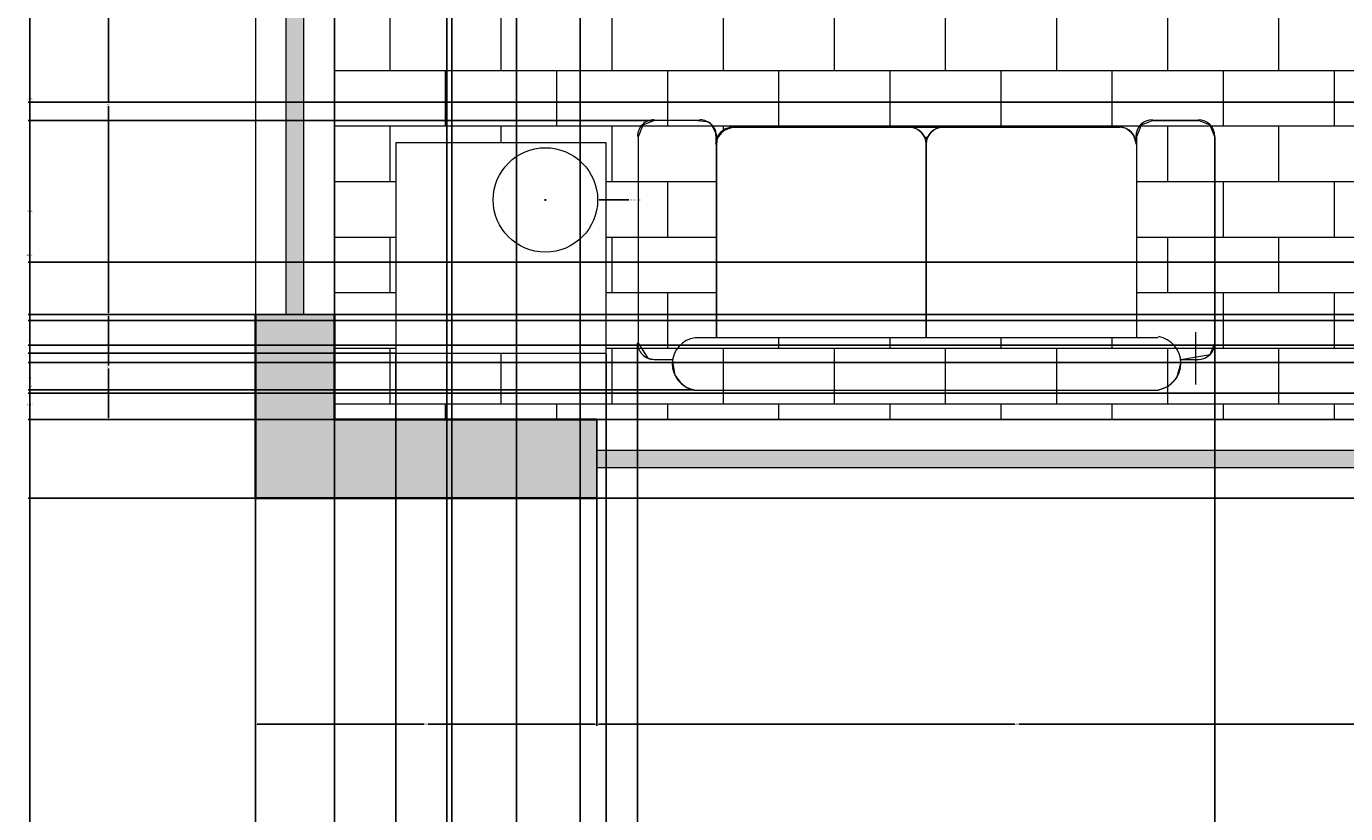
# Model space of a CAD drawing. Units: inches. Extents: x 6 to 575, y 34 to 566.
# Tile 2 of 21: x 6 to 157, y 168 to 258. Entities that reach past the tile are written whole.
import ezdxf

# ---------------------------------------------------------------- set-up
doc = ezdxf.new("R2010")
doc.units = ezdxf.units.IN
for name, color, linetype, lineweight in [('A-ANNO-DIMS', 2, 'Continuous', 18), ('A-FLOR-PATT', 252, 'Continuous', 9), ('A-GLAZ-PATT', 4, 'Continuous', 9), ('A-WALL-PATT', 251, 'Continuous', 9), ('FUR', 2, 'Continuous', 18), ('WALLS', 7, 'Continuous', 35), ('WINDOWS', 4, 'Continuous', 20)]:
    doc.layers.add(name, color=color, linetype=linetype, lineweight=lineweight)
doc.styles.get("Standard").update_dxf_attribs({"font": 'arial.ttf'})
doc.dimstyles.get("Standard").update_dxf_attribs({"dimtxt": 0.18, "dimasz": 0.18, "dimexe": 0.18, "dimexo": 0.0625, "dimgap": 0.09, "dimtad": 0, "dimtih": 1, "dimtoh": 1, "dimdec": 4, "dimzin": 0, "dimdsep": 46, "dimtxsty": 'Standard', "dimcen": 0.09, "dimadec": 0, "dimazin": 0, "dimtfac": 1, "dimtdec": 4, "dimtofl": 0, "dimtmove": 0, "dimatfit": 3, "dimfxl": 1, "dimtolj": 1, "dimtzin": 0, "dimarcsym": 0})

# ---------------------------------------------------------------- blocks, each defined once
blk = doc.blocks.new('*D29')
at = {"layer": 'A-ANNO-DIMS', "color": 0, "lineweight": -2, "transparency": 16777216}
for p, q in [((32.66, 203.74), (32.66, 33.76)), ((548.66, 203.74), (548.66, 33.76)), ((32.84, 33.94), (290.37, 33.94)), ((548.48, 33.94), (290.95, 33.94))]:
    blk.add_line(p, q, dxfattribs=at)
at = {"layer": 'A-ANNO-DIMS', "color": 0, "transparency": 16777216}
for points in [[(32.84, 33.97), (32.84, 33.91), (32.66, 33.94)], [(548.48, 33.97), (548.48, 33.91), (548.66, 33.94)]]:
    blk.add_solid(points, dxfattribs=at)
at = {"layer": 'Defpoints', "color": 0, "transparency": 16777216}
for p in [(32.66, 203.8), (548.66, 203.8), (548.66, 33.94)]:
    blk.add_point(p, dxfattribs=at)
at = {"layer": 'A-ANNO-DIMS', "color": 0, "transparency": 16777216, "insert": (290.66, 33.94), "char_height": 0.18, "attachment_point": 5}
blk.add_mtext('\\A1;516', dxfattribs=at)
blk = doc.blocks.new('*D30')
at = {"layer": 'A-ANNO-DIMS', "color": 0, "lineweight": -2, "transparency": 16777216}
for p, q in [((32.6, 539.8), (6.65, 539.8)), ((6.83, 539.62), (6.83, 299.97)), ((6.83, 59.95), (6.83, 299.61)), ((197.62, 59.77), (6.65, 59.77))]:
    blk.add_line(p, q, dxfattribs=at)
at = {"layer": 'A-ANNO-DIMS', "color": 0, "transparency": 16777216}
for points in [[(6.8, 539.62), (6.86, 539.62), (6.83, 539.8)], [(6.8, 59.95), (6.86, 59.95), (6.83, 59.77)]]:
    blk.add_solid(points, dxfattribs=at)
at = {"layer": 'Defpoints', "color": 0, "transparency": 16777216}
for p in [(32.66, 539.8), (6.83, 59.77), (197.69, 59.77)]:
    blk.add_point(p, dxfattribs=at)
at = {"layer": 'A-ANNO-DIMS', "color": 0, "transparency": 16777216, "insert": (6.83, 299.79), "char_height": 0.18, "attachment_point": 5}
blk.add_mtext('\\A1;480', dxfattribs=at)
blk = doc.blocks.new('*D37')
at = {"layer": 'A-ANNO-DIMS', "color": 0, "lineweight": -2, "transparency": 16777216}
for p, q in [((71.66, 203.74), (71.66, 177.79)), ((167.66, 203.74), (167.66, 177.79)), ((71.84, 177.97), (119.44, 177.97)), ((167.48, 177.97), (119.88, 177.97))]:
    blk.add_line(p, q, dxfattribs=at)
at = {"layer": 'A-ANNO-DIMS', "color": 0, "transparency": 16777216}
for points in [[(71.84, 178), (71.84, 177.94), (71.66, 177.97)], [(167.48, 178), (167.48, 177.94), (167.66, 177.97)]]:
    blk.add_solid(points, dxfattribs=at)
at = {"layer": 'Defpoints', "color": 0, "transparency": 16777216}
for p in [(71.66, 203.8), (167.66, 203.8), (71.66, 177.97)]:
    blk.add_point(p, dxfattribs=at)
at = {"layer": 'A-ANNO-DIMS', "color": 0, "transparency": 16777216, "insert": (119.66, 177.97), "char_height": 0.18, "attachment_point": 5}
blk.add_mtext('\\A1;96', dxfattribs=at)
blk = doc.blocks.new('*D38')
at = {"layer": 'A-ANNO-DIMS', "color": 0, "lineweight": -2, "transparency": 16777216}
for p, q in [((32.66, 203.74), (32.66, 177.79)), ((71.66, 203.74), (71.66, 177.79)), ((32.84, 177.97), (51.94, 177.97)), ((71.48, 177.97), (52.38, 177.97))]:
    blk.add_line(p, q, dxfattribs=at)
at = {"layer": 'A-ANNO-DIMS', "color": 0, "transparency": 16777216}
for points in [[(32.84, 178), (32.84, 177.94), (32.66, 177.97)], [(71.48, 178), (71.48, 177.94), (71.66, 177.97)]]:
    blk.add_solid(points, dxfattribs=at)
at = {"layer": 'Defpoints', "color": 0, "transparency": 16777216}
for p in [(32.66, 203.8), (71.66, 203.8), (32.66, 177.97)]:
    blk.add_point(p, dxfattribs=at)
at = {"layer": 'A-ANNO-DIMS', "color": 0, "transparency": 16777216, "insert": (52.16, 177.97), "char_height": 0.18, "attachment_point": 5}
blk.add_mtext('\\A1;39', dxfattribs=at)
blk = doc.blocks.new('*D42')
at = {"layer": 'A-ANNO-DIMS', "color": 0, "lineweight": -2, "transparency": 16777216}
for p, q in [((41.6, 224.8), (15.65, 224.8)), ((15.83, 224.62), (15.83, 218.98)), ((15.83, 212.98), (15.83, 218.62)), ((41.6, 212.8), (15.65, 212.8))]:
    blk.add_line(p, q, dxfattribs=at)
at = {"layer": 'A-ANNO-DIMS', "color": 0, "transparency": 16777216}
for points in [[(15.8, 224.62), (15.86, 224.62), (15.83, 224.8)], [(15.8, 212.98), (15.86, 212.98), (15.83, 212.8)]]:
    blk.add_solid(points, dxfattribs=at)
at = {"layer": 'Defpoints', "color": 0, "transparency": 16777216}
for p in [(15.83, 224.8), (41.66, 224.8), (41.66, 212.8)]:
    blk.add_point(p, dxfattribs=at)
at = {"layer": 'A-ANNO-DIMS', "color": 0, "transparency": 16777216, "insert": (15.83, 218.8), "char_height": 0.18, "attachment_point": 5}
blk.add_mtext('\\A1;12', dxfattribs=at)
blk = doc.blocks.new('*D43')
at = {"layer": 'A-ANNO-DIMS', "color": 0, "lineweight": -2, "transparency": 16777216}
for p, q in [((41.6, 272.8), (15.65, 272.8)), ((15.83, 272.62), (15.83, 248.98)), ((15.83, 224.98), (15.83, 248.62)), ((41.6, 224.8), (15.65, 224.8))]:
    blk.add_line(p, q, dxfattribs=at)
at = {"layer": 'A-ANNO-DIMS', "color": 0, "transparency": 16777216}
for points in [[(15.8, 272.62), (15.86, 272.62), (15.83, 272.8)], [(15.8, 224.98), (15.86, 224.98), (15.83, 224.8)]]:
    blk.add_solid(points, dxfattribs=at)
at = {"layer": 'Defpoints', "color": 0, "transparency": 16777216}
for p in [(15.83, 272.8), (41.66, 272.8), (41.66, 224.8)]:
    blk.add_point(p, dxfattribs=at)
at = {"layer": 'A-ANNO-DIMS', "color": 0, "transparency": 16777216, "insert": (15.83, 248.8), "char_height": 0.18, "attachment_point": 5}
blk.add_mtext('\\A1;48', dxfattribs=at)
blk = doc.blocks.new('*D77')
at = {"layer": 'A-ANNO-DIMS', "color": 0, "lineweight": -2, "transparency": 16777216}
for p, q in [((197.62, 203.8), (6.65, 203.8)), ((6.83, 203.62), (6.83, 131.97)), ((6.83, 59.95), (6.83, 131.61)), ((197.62, 59.77), (6.65, 59.77))]:
    blk.add_line(p, q, dxfattribs=at)
at = {"layer": 'A-ANNO-DIMS', "color": 0, "transparency": 16777216}
for points in [[(6.8, 203.62), (6.86, 203.62), (6.83, 203.8)], [(6.8, 59.95), (6.86, 59.95), (6.83, 59.77)]]:
    blk.add_solid(points, dxfattribs=at)
at = {"layer": 'Defpoints', "color": 0, "transparency": 16777216}
for p in [(6.83, 203.8), (197.69, 203.8), (197.69, 59.77)]:
    blk.add_point(p, dxfattribs=at)
at = {"layer": 'A-ANNO-DIMS', "color": 0, "transparency": 16777216, "insert": (6.83, 131.79), "char_height": 0.18, "attachment_point": 5}
blk.add_mtext('\\A1;144.03', dxfattribs=at)
blk = doc.blocks.new('*D90')
at = {"layer": 'A-ANNO-DIMS', "color": 0, "lineweight": -2, "transparency": 16777216}
for p, q in [((41.6, 286.06), (6.65, 286.06)), ((6.83, 285.88), (6.83, 249.61)), ((6.83, 212.98), (6.83, 249.25)), ((41.6, 212.8), (6.65, 212.8))]:
    blk.add_line(p, q, dxfattribs=at)
at = {"layer": 'A-ANNO-DIMS', "color": 0, "transparency": 16777216}
for points in [[(6.8, 285.88), (6.86, 285.88), (6.83, 286.06)], [(6.8, 212.98), (6.86, 212.98), (6.83, 212.8)]]:
    blk.add_solid(points, dxfattribs=at)
at = {"layer": 'Defpoints', "color": 0, "transparency": 16777216}
for p in [(6.83, 286.06), (41.66, 286.06), (41.66, 212.8)]:
    blk.add_point(p, dxfattribs=at)
at = {"layer": 'A-ANNO-DIMS', "color": 0, "transparency": 16777216, "insert": (6.83, 249.43), "char_height": 0.18, "attachment_point": 5}
blk.add_mtext('\\A1;73.26', dxfattribs=at)
blk = doc.blocks.new('*D91')
at = {"layer": 'A-ANNO-DIMS', "color": 0, "lineweight": -2, "transparency": 16777216}
for p, q in [((62.49, 286), (62.49, 33.76)), ((41.66, 265.01), (41.66, 33.76)), ((41.84, 33.94), (51.68, 33.94)), ((62.31, 33.94), (52.47, 33.94))]:
    blk.add_line(p, q, dxfattribs=at)
at = {"layer": 'A-ANNO-DIMS', "color": 0, "transparency": 16777216}
for points in [[(41.84, 33.97), (41.84, 33.91), (41.66, 33.94)], [(62.31, 33.97), (62.31, 33.91), (62.49, 33.94)]]:
    blk.add_solid(points, dxfattribs=at)
at = {"layer": 'Defpoints', "color": 0, "transparency": 16777216}
for p in [(62.49, 286.06), (41.66, 265.08), (62.49, 33.94)]:
    blk.add_point(p, dxfattribs=at)
at = {"layer": 'A-ANNO-DIMS', "color": 0, "transparency": 16777216, "insert": (52.07, 33.94), "char_height": 0.18, "attachment_point": 5}
blk.add_mtext('\\A1;20.83', dxfattribs=at)
blk = doc.blocks.new('*D93')
at = {"layer": 'A-ANNO-DIMS', "color": 0, "lineweight": -2, "transparency": 16777216}
for p, q in [((54.53, 298.17), (54.53, 33.76)), ((69.75, 298.17), (69.75, 33.76)), ((54.71, 33.94), (61.68, 33.94)), ((69.57, 33.94), (62.59, 33.94))]:
    blk.add_line(p, q, dxfattribs=at)
at = {"layer": 'A-ANNO-DIMS', "color": 0, "transparency": 16777216}
for points in [[(54.71, 33.97), (54.71, 33.91), (54.53, 33.94)], [(69.57, 33.97), (69.57, 33.91), (69.75, 33.94)]]:
    blk.add_solid(points, dxfattribs=at)
at = {"layer": 'Defpoints', "color": 0, "transparency": 16777216}
for p in [(54.53, 298.24), (69.75, 298.24), (69.75, 33.94)]:
    blk.add_point(p, dxfattribs=at)
at = {"layer": 'A-ANNO-DIMS', "color": 0, "transparency": 16777216, "insert": (62.14, 33.94), "char_height": 0.18, "attachment_point": 5}
blk.add_mtext('\\A1;15.214', dxfattribs=at)
blk = doc.blocks.new('*D97')
at = {"layer": 'A-ANNO-DIMS', "color": 0, "lineweight": -2, "transparency": 16777216}
for p, q in [((55.08, 297.86), (55.08, 33.76)), ((41.66, 286), (41.66, 33.76)), ((41.84, 33.94), (47.98, 33.94)), ((54.9, 33.94), (48.75, 33.94))]:
    blk.add_line(p, q, dxfattribs=at)
at = {"layer": 'A-ANNO-DIMS', "color": 0, "transparency": 16777216}
for points in [[(41.84, 33.97), (41.84, 33.91), (41.66, 33.94)], [(54.9, 33.97), (54.9, 33.91), (55.08, 33.94)]]:
    blk.add_solid(points, dxfattribs=at)
at = {"layer": 'Defpoints', "color": 0, "transparency": 16777216}
for p in [(55.08, 297.92), (41.66, 286.06), (55.08, 33.94)]:
    blk.add_point(p, dxfattribs=at)
at = {"layer": 'A-ANNO-DIMS', "color": 0, "transparency": 16777216, "insert": (48.37, 33.94), "char_height": 0.18, "attachment_point": 5}
blk.add_mtext('\\A1;13.42', dxfattribs=at)
blk = doc.blocks.new('*D98')
at = {"layer": 'A-ANNO-DIMS', "color": 0, "lineweight": -2, "transparency": 16777216}
for p, q in [((48.68, 220.31), (48.68, 33.76)), ((41.66, 212.74), (41.66, 33.76)), ((41.84, 33.94), (44.78, 33.94)), ((48.5, 33.94), (45.56, 33.94))]:
    blk.add_line(p, q, dxfattribs=at)
at = {"layer": 'A-ANNO-DIMS', "color": 0, "transparency": 16777216}
for points in [[(41.84, 33.97), (41.84, 33.91), (41.66, 33.94)], [(48.5, 33.97), (48.5, 33.91), (48.68, 33.94)]]:
    blk.add_solid(points, dxfattribs=at)
at = {"layer": 'Defpoints', "color": 0, "transparency": 16777216}
for p in [(48.68, 220.37), (41.66, 212.8), (48.68, 33.94)]:
    blk.add_point(p, dxfattribs=at)
at = {"layer": 'A-ANNO-DIMS', "color": 0, "transparency": 16777216, "insert": (45.17, 33.94), "char_height": 0.18, "attachment_point": 5}
blk.add_mtext('\\A1;7.022', dxfattribs=at)
blk = doc.blocks.new('*D99')
at = {"layer": 'A-ANNO-DIMS', "color": 0, "lineweight": -2, "transparency": 16777216}
for p, q in [((48.62, 220.37), (6.65, 220.37)), ((6.83, 220.19), (6.83, 216.77)), ((6.83, 212.98), (6.83, 216.4)), ((41.6, 212.8), (6.65, 212.8))]:
    blk.add_line(p, q, dxfattribs=at)
at = {"layer": 'A-ANNO-DIMS', "color": 0, "transparency": 16777216}
for points in [[(6.8, 220.19), (6.86, 220.19), (6.83, 220.37)], [(6.8, 212.98), (6.86, 212.98), (6.83, 212.8)]]:
    blk.add_solid(points, dxfattribs=at)
at = {"layer": 'Defpoints', "color": 0, "transparency": 16777216}
for p in [(6.83, 220.37), (48.68, 220.37), (41.66, 212.8)]:
    blk.add_point(p, dxfattribs=at)
at = {"layer": 'A-ANNO-DIMS', "color": 0, "transparency": 16777216, "insert": (6.83, 216.59), "char_height": 0.18, "attachment_point": 5}
blk.add_mtext('\\A1;7.571', dxfattribs=at)
blk = doc.blocks.new('*D100')
at = {"layer": 'A-ANNO-DIMS', "color": 0, "lineweight": -2, "transparency": 16777216}
for p, q in [((72.71, 220.31), (72.71, 33.76)), ((76.3, 221.52), (76.3, 33.76)), ((72.89, 33.94), (74.11, 33.94)), ((76.12, 33.94), (74.9, 33.94))]:
    blk.add_line(p, q, dxfattribs=at)
at = {"layer": 'A-ANNO-DIMS', "color": 0, "transparency": 16777216}
for points in [[(72.89, 33.97), (72.89, 33.91), (72.71, 33.94)], [(76.12, 33.97), (76.12, 33.91), (76.3, 33.94)]]:
    blk.add_solid(points, dxfattribs=at)
at = {"layer": 'Defpoints', "color": 0, "transparency": 16777216}
for p in [(72.71, 220.37), (76.3, 221.58), (76.3, 33.94)]:
    blk.add_point(p, dxfattribs=at)
at = {"layer": 'A-ANNO-DIMS', "color": 0, "transparency": 16777216, "insert": (74.5, 33.94), "char_height": 0.18, "attachment_point": 5}
blk.add_mtext('\\A1;3.589', dxfattribs=at)
blk = doc.blocks.new('*D101')
at = {"layer": 'A-ANNO-DIMS', "color": 0, "lineweight": -2, "transparency": 16777216}
for p, q in [((76.3, 221.52), (76.3, 33.76)), ((142.3, 221.48), (142.3, 33.76)), ((76.48, 33.94), (109.08, 33.94)), ((142.12, 33.94), (109.52, 33.94))]:
    blk.add_line(p, q, dxfattribs=at)
at = {"layer": 'A-ANNO-DIMS', "color": 0, "transparency": 16777216}
for points in [[(76.48, 33.97), (76.48, 33.91), (76.3, 33.94)], [(142.12, 33.97), (142.12, 33.91), (142.3, 33.94)]]:
    blk.add_solid(points, dxfattribs=at)
at = {"layer": 'Defpoints', "color": 0, "transparency": 16777216}
for p in [(76.3, 221.58), (142.3, 221.54), (142.3, 33.94)]:
    blk.add_point(p, dxfattribs=at)
at = {"layer": 'A-ANNO-DIMS', "color": 0, "transparency": 16777216, "insert": (109.3, 33.94), "char_height": 0.18, "attachment_point": 5}
blk.add_mtext('\\A1;66', dxfattribs=at)
blk = doc.blocks.new('*D102')
at = {"layer": 'A-ANNO-DIMS', "color": 0, "lineweight": -2, "transparency": 16777216}
for p, q in [((78.19, 246.98), (6.65, 246.98)), ((6.83, 246.8), (6.83, 231.77)), ((6.83, 216.38), (6.83, 231.41)), ((82.72, 216.2), (6.65, 216.2))]:
    blk.add_line(p, q, dxfattribs=at)
at = {"layer": 'A-ANNO-DIMS', "color": 0, "transparency": 16777216}
for points in [[(6.8, 246.8), (6.86, 246.8), (6.83, 246.98)], [(6.8, 216.38), (6.86, 216.38), (6.83, 216.2)]]:
    blk.add_solid(points, dxfattribs=at)
at = {"layer": 'Defpoints', "color": 0, "transparency": 16777216}
for p in [(78.25, 246.98), (6.83, 216.2), (82.79, 216.2)]:
    blk.add_point(p, dxfattribs=at)
at = {"layer": 'A-ANNO-DIMS', "color": 0, "transparency": 16777216, "insert": (6.83, 231.59), "char_height": 0.18, "attachment_point": 5}
blk.add_mtext('\\A1;30.777', dxfattribs=at)
blk = doc.blocks.new('*D103')
at = {"layer": 'A-ANNO-DIMS', "color": 0, "lineweight": -2, "transparency": 16777216}
for p, q in [((82.72, 216.2), (6.65, 216.2)), ((6.83, 216.02), (6.83, 214.68)), ((6.83, 212.98), (6.83, 214.32)), ((71.6, 212.8), (6.65, 212.8))]:
    blk.add_line(p, q, dxfattribs=at)
at = {"layer": 'A-ANNO-DIMS', "color": 0, "transparency": 16777216}
for points in [[(6.8, 216.02), (6.86, 216.02), (6.83, 216.2)], [(6.8, 212.98), (6.86, 212.98), (6.83, 212.8)]]:
    blk.add_solid(points, dxfattribs=at)
at = {"layer": 'Defpoints', "color": 0, "transparency": 16777216}
for p in [(82.79, 216.2), (6.83, 212.8), (71.66, 212.8)]:
    blk.add_point(p, dxfattribs=at)
at = {"layer": 'A-ANNO-DIMS', "color": 0, "transparency": 16777216, "insert": (6.83, 214.5), "char_height": 0.18, "attachment_point": 5}
blk.add_mtext('\\A1;3.399', dxfattribs=at)
blk = doc.blocks.new('*D107')
at = {"layer": 'A-ANNO-DIMS', "color": 0, "lineweight": -2, "transparency": 16777216}
for p, q in [((197.6, 230.8), (6.65, 230.8)), ((6.83, 230.62), (6.83, 221.98)), ((6.83, 212.98), (6.83, 221.62)), ((197.6, 212.8), (6.65, 212.8))]:
    blk.add_line(p, q, dxfattribs=at)
at = {"layer": 'A-ANNO-DIMS', "color": 0, "transparency": 16777216}
for points in [[(6.8, 230.62), (6.86, 230.62), (6.83, 230.8)], [(6.8, 212.98), (6.86, 212.98), (6.83, 212.8)]]:
    blk.add_solid(points, dxfattribs=at)
at = {"layer": 'Defpoints', "color": 0, "transparency": 16777216}
for p in [(6.83, 230.8), (197.66, 230.8), (197.66, 212.8)]:
    blk.add_point(p, dxfattribs=at)
at = {"layer": 'A-ANNO-DIMS', "color": 0, "transparency": 16777216, "insert": (6.83, 221.8), "char_height": 0.18, "attachment_point": 5}
blk.add_mtext('\\A1;18', dxfattribs=at)
blk = doc.blocks.new('*D108')
at = {"layer": 'A-ANNO-DIMS', "color": 0, "lineweight": -2, "transparency": 16777216}
for p, q in [((197.6, 276.8), (6.65, 276.8)), ((6.83, 276.62), (6.83, 253.98)), ((6.83, 230.98), (6.83, 253.62)), ((197.6, 230.8), (6.65, 230.8))]:
    blk.add_line(p, q, dxfattribs=at)
at = {"layer": 'A-ANNO-DIMS', "color": 0, "transparency": 16777216}
for points in [[(6.8, 276.62), (6.86, 276.62), (6.83, 276.8)], [(6.8, 230.98), (6.86, 230.98), (6.83, 230.8)]]:
    blk.add_solid(points, dxfattribs=at)
at = {"layer": 'Defpoints', "color": 0, "transparency": 16777216}
for p in [(6.83, 276.8), (197.66, 276.8), (197.66, 230.8)]:
    blk.add_point(p, dxfattribs=at)
at = {"layer": 'A-ANNO-DIMS', "color": 0, "transparency": 16777216, "insert": (6.83, 253.8), "char_height": 0.18, "attachment_point": 5}
blk.add_mtext('\\A1;46', dxfattribs=at)
blk = doc.blocks.new('*D137')
at = {"layer": 'A-ANNO-DIMS', "color": 0, "lineweight": -2, "transparency": 16777216}
for p, q in [((206.62, 310.57), (6.65, 310.57)), ((6.83, 310.39), (6.83, 267.87)), ((6.83, 224.98), (6.83, 267.5)), ((206.6, 224.8), (6.65, 224.8))]:
    blk.add_line(p, q, dxfattribs=at)
at = {"layer": 'A-ANNO-DIMS', "color": 0, "transparency": 16777216}
for points in [[(6.8, 310.39), (6.86, 310.39), (6.83, 310.57)], [(6.8, 224.98), (6.86, 224.98), (6.83, 224.8)]]:
    blk.add_solid(points, dxfattribs=at)
at = {"layer": 'Defpoints', "color": 0, "transparency": 16777216}
for p in [(6.83, 310.57), (206.68, 310.57), (206.66, 224.8)]:
    blk.add_point(p, dxfattribs=at)
at = {"layer": 'A-ANNO-DIMS', "color": 0, "transparency": 16777216, "insert": (6.83, 267.69), "char_height": 0.18, "attachment_point": 5}
blk.add_mtext('\\A1;85.77', dxfattribs=at)
blk = doc.blocks.new('*D209')
at = {"layer": 'A-ANNO-DIMS', "color": 0, "lineweight": -2, "transparency": 16777216}
for p, q in [((265.64, 249.08), (6.65, 249.08)), ((6.83, 248.9), (6.83, 236.78)), ((6.83, 224.3), (6.83, 236.42)), ((265.64, 224.12), (6.65, 224.12))]:
    blk.add_line(p, q, dxfattribs=at)
at = {"layer": 'A-ANNO-DIMS', "color": 0, "transparency": 16777216}
for points in [[(6.8, 248.9), (6.86, 248.9), (6.83, 249.08)], [(6.8, 224.3), (6.86, 224.3), (6.83, 224.12)]]:
    blk.add_solid(points, dxfattribs=at)
at = {"layer": 'Defpoints', "color": 0, "transparency": 16777216}
for p in [(6.83, 249.08), (265.7, 249.08), (265.7, 224.12)]:
    blk.add_point(p, dxfattribs=at)
at = {"layer": 'A-ANNO-DIMS', "color": 0, "transparency": 16777216, "insert": (6.83, 236.6), "char_height": 0.18, "attachment_point": 5}
blk.add_mtext('\\A1;24.96', dxfattribs=at)
blk = doc.blocks.new('*D214')
at = {"layer": 'A-ANNO-DIMS', "color": 0, "lineweight": -2, "transparency": 16777216}
for p, q in [((246.6, 219.3), (6.65, 219.3)), ((6.83, 219.12), (6.83, 217.73)), ((6.83, 215.98), (6.83, 217.37)), ((246.6, 215.8), (6.65, 215.8))]:
    blk.add_line(p, q, dxfattribs=at)
at = {"layer": 'A-ANNO-DIMS', "color": 0, "transparency": 16777216}
for points in [[(6.8, 219.12), (6.86, 219.12), (6.83, 219.3)], [(6.8, 215.98), (6.86, 215.98), (6.83, 215.8)]]:
    blk.add_solid(points, dxfattribs=at)
at = {"layer": 'Defpoints', "color": 0, "transparency": 16777216}
for p in [(6.83, 219.3), (246.66, 219.3), (246.66, 215.8)]:
    blk.add_point(p, dxfattribs=at)
at = {"layer": 'A-ANNO-DIMS', "color": 0, "transparency": 16777216, "insert": (6.83, 217.55), "char_height": 0.18, "attachment_point": 5}
blk.add_mtext('\\A1;3.5', dxfattribs=at)
blk = doc.blocks.new('*D215')
at = {"layer": 'A-ANNO-DIMS', "color": 0, "lineweight": -2, "transparency": 16777216}
for p, q in [((246.6, 221.3), (6.65, 221.3)), ((6.83, 221.12), (6.83, 220.48)), ((246.6, 219.3), (6.65, 219.3)), ((6.83, 219.48), (6.83, 220.12))]:
    blk.add_line(p, q, dxfattribs=at)
at = {"layer": 'A-ANNO-DIMS', "color": 0, "transparency": 16777216}
for points in [[(6.8, 221.12), (6.86, 221.12), (6.83, 221.3)], [(6.8, 219.48), (6.86, 219.48), (6.83, 219.3)]]:
    blk.add_solid(points, dxfattribs=at)
at = {"layer": 'Defpoints', "color": 0, "transparency": 16777216}
for p in [(6.83, 221.3), (246.66, 221.3), (246.66, 219.3)]:
    blk.add_point(p, dxfattribs=at)
at = {"layer": 'A-ANNO-DIMS', "color": 0, "transparency": 16777216, "insert": (6.83, 220.3), "char_height": 0.18, "attachment_point": 5}
blk.add_mtext('\\A1;2', dxfattribs=at)
blk = doc.blocks.new('*D243')
at = {"layer": 'A-ANNO-DIMS', "color": 0, "lineweight": -2, "transparency": 16777216}
for p, q in [((65.69, 237.9), (65.87, 237.9)), ((65.78, 237.81), (65.78, 237.99)), ((75.33, 237.89), (71.93, 237.89))]:
    blk.add_line(p, q, dxfattribs=at)
at = {"layer": 'A-ANNO-DIMS', "color": 0, "transparency": 16777216}
blk.add_solid([(71.93, 237.92), (71.93, 237.86), (71.75, 237.89)], dxfattribs=at)
at = {"layer": 'Defpoints', "color": 0, "transparency": 16777216}
for p in [(59.81, 237.9), (71.75, 237.89)]:
    blk.add_point(p, dxfattribs=at)
at = {"layer": 'A-ANNO-DIMS', "color": 0, "transparency": 16777216, "insert": (76.08, 237.89), "char_height": 0.18, "attachment_point": 5}
blk.add_mtext('\\A1;2X ∅11.937', dxfattribs=at)

msp = doc.modelspace()

# ---------------------------------------------------------------- hatches: boundary and pattern name
at = {"layer": 'A-FLOR-PATT'}
h = msp.add_hatch(dxfattribs=at)
h.set_pattern_fill('BRICK', color=256)
h.set_pattern_definition([(0, (-98.035, 170.1465), (0, 6.35), []), (90, (-98.035, 170.147), (-12.7, 8e-16), [6.35, -6.35]), (90, (-91.685, 170.147), (-12.7, 8e-16), [-6.35, 6.35])])
h.paths.add_polyline_path([(180.8711, 269.7588), (182.4439, 270.6668), (182.4628, 270.6341, -0.11619827), (201.8275, 275.5902), (201.8275, 276.801), (197.6586, 276.801), (197.6586, 293.1641), (182.6401, 293.1641), (182.6401, 348.324), (197.6586, 348.324), (197.6586, 407.7709), (112.8513, 407.7709), (112.8513, 431.801), (111.6586, 431.801), (111.6586, 440.801), (117.6586, 440.801), (117.6586, 446.801), (117.6586, 448.2751), (117.6586, 473.3269), (117.6586, 474.801), (117.6586, 515.5941), (100.2533, 515.5941, -1), (83.0548, 515.5941), (65.6494, 515.5941), (65.6494, 440.801), (82.8918, 440.801), (82.8918, 431.801), (82.8918, 407.7709), (41.6586, 407.7709), (41.6586, 379.0637), (62.6459, 379.0637), (62.6459, 358.0764), (122.565, 358.0764), (122.565, 286.0643), (62.6459, 286.0643), (62.6459, 265.077), (41.6586, 265.077), (41.6586, 224.801), (41.6586, 212.801), (71.6586, 212.801), (167.6586, 212.801), (197.6586, 212.801), (197.6586, 230.801), (201.8157, 230.801), (201.8157, 233.4817)])
h.paths.add_polyline_path([(133.3414, 245.1275), (133.3317, 245.1352), (133.3317, 245.104)], flags=16)
h.paths.add_polyline_path([(133.3317, 222.1662), (85.3496, 222.1662), (85.3496, 243.7443, -0.50090726), (87.1831, 246.1963), (107.4292, 246.1963), (111.2522, 246.1963), (131.4202, 246.1963, -0.41421356), (133.3317, 244.2848)], flags=16)
h.paths.add_polyline_path([(72.7105, 244.4018), (72.7105, 220.3718), (48.6804, 220.3718), (48.6804, 244.4018)], flags=16)
h.paths.add_polyline_path([(71.7466, 237.8955, -1), (59.8096, 237.8955, -1)], flags=0)
at = {"layer": 'A-GLAZ-PATT'}
h = msp.add_hatch(color=256, dxfattribs=at)
h.dxf.hatch_style = 1
h.paths.add_polyline_path([(36.1586, 224.801), (38.1586, 224.801), (38.1586, 272.801), (36.1586, 272.801)])
h.paths.add_polyline_path([(167.6586, 207.301), (167.6586, 209.301), (71.6586, 209.301), (71.6586, 207.301)])
h.paths.add_polyline_path([(264.6586, 219.301), (264.6586, 221.301), (246.6586, 221.301), (246.6586, 219.301)])
h.paths.add_polyline_path([(316.6586, 221.301), (316.6586, 219.301), (334.6586, 219.301), (334.6586, 221.301)])
h.paths.add_polyline_path([(515.6586, 207.301), (515.6586, 209.301), (407.6586, 209.301), (407.6586, 207.301)])
h.paths.add_polyline_path([(543.1586, 270.801), (545.1586, 270.801), (545.1586, 366.801), (543.1586, 366.801)])
h.paths.add_polyline_path([(407.9436, 536.301), (407.9436, 534.301), (455.9436, 534.301), (455.9436, 536.301)])
h.paths.add_polyline_path([(272.6586, 536.301), (272.6586, 534.301), (320.6586, 534.301), (320.6586, 536.301)])
at = {"layer": 'A-WALL-PATT'}
h = msp.add_hatch(color=256, dxfattribs=at)
h.dxf.hatch_style = 1
h.paths.add_polyline_path([(160.6586, 539.801), (32.6586, 539.801), (32.6586, 272.801), (41.6586, 272.801), (41.6586, 286.0643), (41.6586, 358.0764), (41.6586, 379.0637), (41.6586, 407.7709), (41.6194, 407.7709), (41.6194, 431.801), (82.8918, 431.801), (82.8918, 440.801), (65.6494, 440.801), (65.6494, 440.7732), (41.6194, 440.7732), (41.6194, 515.5941), (41.6586, 530.801), (117.6586, 530.801), (117.6586, 474.801), (120.6068, 474.801), (121.6586, 474.801), (121.6586, 530.801), (137.4275, 530.801), (137.4275, 530.8356), (141.2505, 530.8356), (160.6586, 530.801)])
h.paths.add_polyline_path([(71.6586, 212.801), (41.6586, 212.801), (41.6586, 224.801), (32.6586, 224.801), (32.6586, 203.801), (71.6586, 203.801)])
h.paths.add_polyline_path([(206.6586, 215.801), (246.6586, 215.801), (246.6586, 224.801), (206.6586, 224.801), (206.6586, 230.801), (201.8157, 230.801), (197.6586, 230.801), (197.6586, 212.801), (167.6586, 212.801), (167.6586, 203.801), (206.6586, 203.801)])
h.paths.add_polyline_path([(383.6586, 224.801), (334.6586, 224.801), (334.6586, 215.801), (374.6586, 215.801), (374.6586, 203.801), (384.0753, 203.801), (407.6586, 203.801), (407.6586, 212.801), (383.6586, 212.801)])
h.paths.add_polyline_path([(548.6586, 270.801), (539.6586, 270.801), (539.6586, 212.801), (515.6586, 212.801), (515.6586, 203.801), (548.6586, 203.801)])
h.paths.add_polyline_path([(548.6586, 412.801), (545.7108, 412.801), (539.6586, 412.801), (539.6586, 382.801), (433.708, 382.801), (433.708, 378.801), (539.6586, 378.801), (539.6586, 366.801), (548.6586, 366.801)])
h.paths.add_polyline_path([(548.6586, 539.801), (455.9436, 539.801), (455.9436, 530.801), (539.6586, 530.801), (539.6586, 440.801), (548.6586, 440.801)])
h.paths.add_polyline_path([(407.9436, 539.801), (362.6586, 539.801), (362.6586, 530.801), (374.6586, 530.801), (374.6586, 452.801), (354.6586, 452.801), (354.6586, 448.801), (374.6586, 448.801), (374.6586, 278.801), (383.6586, 278.801), (383.6586, 530.801), (407.9436, 530.801)])
h.paths.add_polyline_path([(338.6586, 539.801), (320.6586, 539.801), (320.6586, 530.801), (322.6586, 530.801), (322.6586, 448.801), (326.6586, 448.801), (326.6586, 530.801), (338.6586, 530.801)])
h.paths.add_polyline_path([(272.6586, 539.801), (184.6586, 539.801), (184.6586, 530.801), (197.6586, 530.801), (197.6586, 440.801), (176.6714, 440.801), (121.6586, 440.801), (121.6586, 446.801), (117.6586, 446.801), (117.6586, 440.801), (111.6586, 440.801), (111.6586, 431.801), (197.6586, 431.801), (197.6586, 407.7709), (197.6586, 276.801), (206.6586, 276.801), (206.6586, 530.801), (272.6586, 530.801)])

# ---------------------------------------------------------------- linework, layer by layer
at = {"layer": 'FUR'}
for points in [[(76.3774, 221.5421), (77.4697, 219.8257), (78.2498, 219.6696), (79.2641, 219.6696), (80.2784, 219.6696), (80.5904, 217.8752), (81.2146, 217.017), (81.9168, 216.4708), (82.775, 216.1587), (135.8283, 216.1587), (136.9986, 216.6269), (137.9349, 217.5631), (138.403, 219.2015), (138.403, 219.6696), (141.7578, 220.2158), (142.304, 221.5421), (142.304, 222.6344), (142.304, 224.2728), (142.304, 245.104), (141.7578, 246.4304), (140.4315, 246.9765), (139.8854, 246.9765), (137.7788, 246.9765), (135.2042, 246.9765), (133.8778, 246.4304), (133.3317, 245.104), (133.3317, 244.2458), (133.0196, 245.2601), (132.7856, 245.5721), (132.3955, 245.8842), (132.1614, 246.0403), (131.4592, 246.1963), (87.2221, 246.1963), (86.2859, 245.8842), (85.8958, 245.5721), (85.4277, 244.948), (85.3496, 244.2458), (85.2716, 245.5721), (84.8035, 246.4304), (84.5694, 246.6644), (84.2574, 246.8204), (82.775, 246.9765), (80.9025, 246.9765), (79.2641, 246.9765), (78.2498, 246.9765), (76.9235, 246.4304), (76.3774, 245.104)], [(48.6804, 244.4018), (48.6804, 220.3718), (72.7105, 220.3718), (72.7105, 244.4018)]]:
    msp.add_lwpolyline(points, close=True, dxfattribs=at)
for points in [[(83.4772, 246.9765), (78.2498, 246.9765)], [(87.2221, 246.1963), (107.4292, 246.1963), (111.2522, 246.1963), (131.4592, 246.1963)], [(135.2042, 246.9765), (140.4315, 246.9765)], [(76.3774, 245.104), (76.3774, 221.5421)], [(85.3496, 244.2458), (85.3496, 222.1662), (85.3496, 245.104)], [(109.3017, 222.1662), (109.3017, 244.2458), (109.3017, 222.1662), (109.3017, 245.104)], [(133.3317, 245.104), (133.3317, 222.1662)], [(142.304, 245.104), (142.304, 221.5421)], [(82.931, 222.1662), (135.8283, 222.1662)], [(140.1194, 216.7829), (140.1194, 222.7904)], [(78.2498, 219.6696), (80.2784, 219.6696)], [(138.403, 219.6696), (140.4315, 219.6696)], [(82.775, 216.1587), (135.8283, 216.1587)]]:
    msp.add_lwpolyline(points, dxfattribs=at)
for points in [[(87.1831, 246.1963, 0.4142182), (85.2716, 244.2848, -0.4142182)], [(111.2131, 246.1963, 0.41421073), (109.3017, 244.2848, 0.41421073), (107.3902, 246.1963, -0.41421073), (109.3017, 244.2848, -0.41421073)]]:
    msp.add_lwpolyline(points, format="xyb", close=True, dxfattribs=at)
msp.add_circle((65.7781, 237.8955), 5.9685, dxfattribs=at)
for centre, radius, start, end in [((78.2108, 245.143), 1.9115, 89.999546, 180.000454), ((83.4382, 245.143), 1.9115, 359.999546, 90.000454), ((131.4202, 244.2848), 1.9115, 0.000277, 89.999723), ((135.1652, 245.143), 1.9115, 90.000277, 179.999723), ((140.3925, 245.143), 1.9115, 0.000277, 89.999723), ((83.2822, 219.1624), 3.0038, 97.163798, 260.485857), ((135.3212, 219.2405), 3.0818, 279.690351, 80.309649), ((78.2108, 221.5811), 1.9115, 179.999546, 270.000454), ((140.3925, 221.5811), 1.9115, 270.000277, 359.999723)]:
    msp.add_arc(centre, radius, start, end, dxfattribs=at)
at = {"layer": 'WALLS'}
for p, q in [((32.6586, 203.801), (32.6586, 224.801)), ((41.6586, 212.801), (41.6586, 224.801)), ((71.6586, 212.801), (41.6586, 212.801)), ((71.6586, 203.801), (32.6586, 203.801))]:
    msp.add_line(p, q, dxfattribs=at)
at = {"layer": 'WINDOWS'}
for p, q in [((36.1586, 224.801), (36.1586, 272.801)), ((38.1586, 224.801), (38.1586, 272.801)), ((41.6586, 224.801), (32.6586, 224.801)), ((71.6586, 212.801), (71.6586, 203.801)), ((71.6586, 209.301), (167.6586, 209.301)), ((71.6586, 207.301), (167.6586, 207.301))]:
    msp.add_line(p, q, dxfattribs=at)
for points in [[(32.6586, 224.801), (41.6586, 224.801), (41.6586, 272.801), (32.6586, 272.801)], [(71.6586, 212.801), (167.6586, 212.801), (167.6586, 203.801), (71.6586, 203.801)]]:
    msp.add_lwpolyline(points, close=True, dxfattribs=at)

# ---------------------------------------------------------------- dimensions: what is measured, and where the dimension line sits
at = {"layer": 'A-ANNO-DIMS'}
for base, p1, p2, angle, override, picture, middle in [((6.8286, 59.7747), (32.6586, 539.801), (197.6872, 59.7747), 90, {"dimdec": 0, "dimlfac": 1, "dimrnd": 0, "dimzin": 0, "dimdsep": 46, "dimlunit": 2}, '*D30', (6.8286, 299.7878)), ((6.8286, 310.5712), (206.6586, 224.801), (206.6824, 310.5712), 90, {"dimdec": 2, "dimlfac": 1, "dimrnd": 0, "dimzin": 0, "dimdsep": 46, "dimlunit": 2}, '*D137', (6.8286, 267.6861)), ((6.8286, 286.0643), (41.6586, 212.801), (41.6586, 286.0643), 90, {"dimdec": 2, "dimlfac": 1, "dimrnd": 0, "dimzin": 0, "dimdsep": 46, "dimlunit": 2}, '*D90', (6.8286, 249.4327)), ((6.8286, 276.801), (197.6586, 230.801), (197.6586, 276.801), 90, {"dimdec": 0, "dimlfac": 1, "dimrnd": 0, "dimzin": 0, "dimdsep": 46, "dimlunit": 2}, '*D108', (6.8286, 253.801)), ((15.8286, 272.801), (41.6586, 224.801), (41.6586, 272.801), 90, {"dimdec": 0, "dimlfac": 1, "dimrnd": 0, "dimzin": 0, "dimdsep": 46, "dimlunit": 2}, '*D43', (15.8286, 248.801)), ((6.8286, 249.081), (265.6986, 224.121), (265.6986, 249.081), 90, {"dimdec": 2, "dimlfac": 1, "dimrnd": 0, "dimzin": 0, "dimdsep": 46, "dimlunit": 2}, '*D209', (6.8286, 236.601)), ((6.8286, 216.1999), (78.2498, 246.9765), (82.7857, 216.1999), 90, {"dimdec": 3, "dimlfac": 1, "dimrnd": 0, "dimzin": 0, "dimdsep": 46, "dimlunit": 2}, '*D102', (6.8286, 231.5882)), ((6.8286, 230.801), (197.6586, 212.801), (197.6586, 230.801), 90, {"dimdec": 0, "dimlfac": 1, "dimrnd": 0, "dimzin": 0, "dimdsep": 46, "dimlunit": 2}, '*D107', (6.8286, 221.801)), ((15.8286, 224.801), (41.6586, 212.801), (41.6586, 224.801), 90, {"dimdec": 0, "dimlfac": 1, "dimrnd": 0, "dimzin": 0, "dimdsep": 46, "dimlunit": 2}, '*D42', (15.8286, 218.801)), ((6.8286, 220.3718), (41.6586, 212.801), (48.6804, 220.3718), 90, {"dimdec": 3, "dimlfac": 1, "dimrnd": 0, "dimzin": 0, "dimdsep": 46, "dimlunit": 2}, '*D99', (6.8286, 216.5864)), ((6.8286, 221.301), (246.6586, 219.301), (246.6586, 221.301), 90, {"dimdec": 0, "dimlfac": 1, "dimrnd": 0, "dimzin": 0, "dimdsep": 46, "dimlunit": 2}, '*D215', (6.8286, 220.301)), ((6.8286, 219.301), (246.6586, 215.801), (246.6586, 219.301), 90, {"dimdec": 1, "dimlfac": 1, "dimrnd": 0, "dimzin": 0, "dimdsep": 46, "dimlunit": 2}, '*D214', (6.8286, 217.551)), ((6.8286, 212.801), (82.7857, 216.1999), (71.6586, 212.801), 90, {"dimdec": 3, "dimlfac": 1, "dimrnd": 0, "dimzin": 0, "dimdsep": 46, "dimlunit": 2}, '*D103', (6.8286, 214.5005)), ((6.8286, 203.801), (197.6872, 59.7747), (197.6864, 203.801), 90, {"dimdec": 2, "dimlfac": 1, "dimrnd": 0, "dimzin": 0, "dimdsep": 46, "dimlunit": 2}, '*D77', (6.8286, 131.7878)), ((32.6586, 177.971), (71.6586, 203.801), (32.6586, 203.801), 180, {"dimdec": 0, "dimlfac": 1, "dimrnd": 0, "dimzin": 0, "dimdsep": 46, "dimlunit": 2}, '*D38', (52.1586, 177.971)), ((71.6586, 177.971), (167.6586, 203.801), (71.6586, 203.801), 180, {"dimdec": 0, "dimlfac": 1, "dimrnd": 0, "dimzin": 0, "dimdsep": 46, "dimlunit": 2}, '*D37', (119.6586, 177.971))]:
    dim = msp.add_linear_dim(base=base, p1=p1, p2=p2, angle=angle, dimstyle='Standard', override=override, dxfattribs=at)
    dim.commit()
    dim.dimension.update_dxf_attribs({"geometry": picture, "text_midpoint": middle})
for base, p1, p2, override, picture, middle in [((55.078, 33.9447), (41.6586, 286.0643), (55.078, 297.9233), {"dimdec": 2, "dimlfac": 1, "dimrnd": 0, "dimzin": 0, "dimdsep": 46, "dimlunit": 2}, '*D97', (48.3683, 33.9447)), ((69.7457, 33.9447), (54.5319, 298.2354), (69.7457, 298.2354), {"dimdec": 3, "dimlfac": 1, "dimrnd": 0, "dimzin": 0, "dimdsep": 46, "dimlunit": 2}, '*D93', (62.1388, 33.9447)), ((62.4899, 33.9447), (41.6586, 265.077), (62.4899, 286.0643), {"dimdec": 2, "dimlfac": 1, "dimrnd": 0, "dimzin": 0, "dimdsep": 46, "dimlunit": 2}, '*D91', (52.0743, 33.9447)), ((48.6804, 33.9447), (41.6586, 212.801), (48.6804, 220.3718), {"dimdec": 3, "dimlfac": 1, "dimrnd": 0, "dimzin": 0, "dimdsep": 46, "dimlunit": 2}, '*D98', (45.1695, 33.9447)), ((76.2994, 33.9447), (72.7105, 220.3718), (76.2994, 221.5811), {"dimdec": 3, "dimlfac": 1, "dimrnd": 0, "dimzin": 0, "dimdsep": 46, "dimlunit": 2}, '*D100', (74.5049, 33.9447)), ((142.304, 33.9447), (76.2994, 221.5811), (142.304, 221.5421), {"dimdec": 0, "dimlfac": 1, "dimrnd": 0, "dimzin": 0, "dimdsep": 46, "dimlunit": 2}, '*D101', (109.3017, 33.9447)), ((548.6586, 33.9447), (32.6586, 203.801), (548.6586, 203.801), {"dimdec": 0, "dimlfac": 1, "dimrnd": 0, "dimzin": 0, "dimdsep": 46, "dimlunit": 2}, '*D29', (290.6586, 33.9447))]:
    dim = msp.add_linear_dim(base=base, p1=p1, p2=p2, dimstyle='Standard', override=override, dxfattribs=at)
    dim.commit()
    dim.dimension.update_dxf_attribs({"geometry": picture, "text_midpoint": middle})
dim = msp.add_diameter_dim_2p(p1=(59.8096, 237.8959), p2=(71.7466, 237.895), text='2X <>', dimstyle='Standard', override={"dimdec": 3, "dimlfac": 1, "dimrnd": 0, "dimzin": 0, "dimdsep": 46, "dimlunit": 2}, dxfattribs=at)
dim.commit()
dim.dimension.update_dxf_attribs({"geometry": '*D243', "text_midpoint": (75.3277, 237.8947), "dimtype": 163})

doc.saveas('drawing.dxf')
